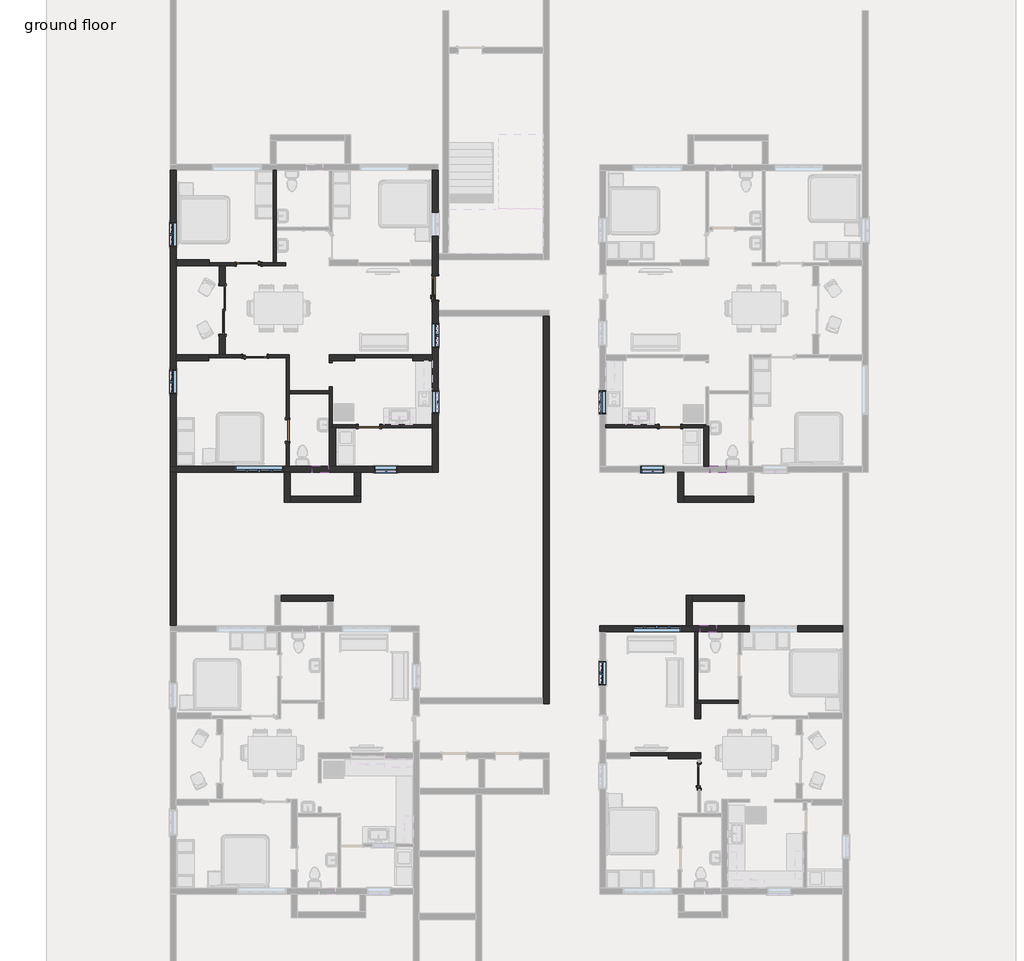
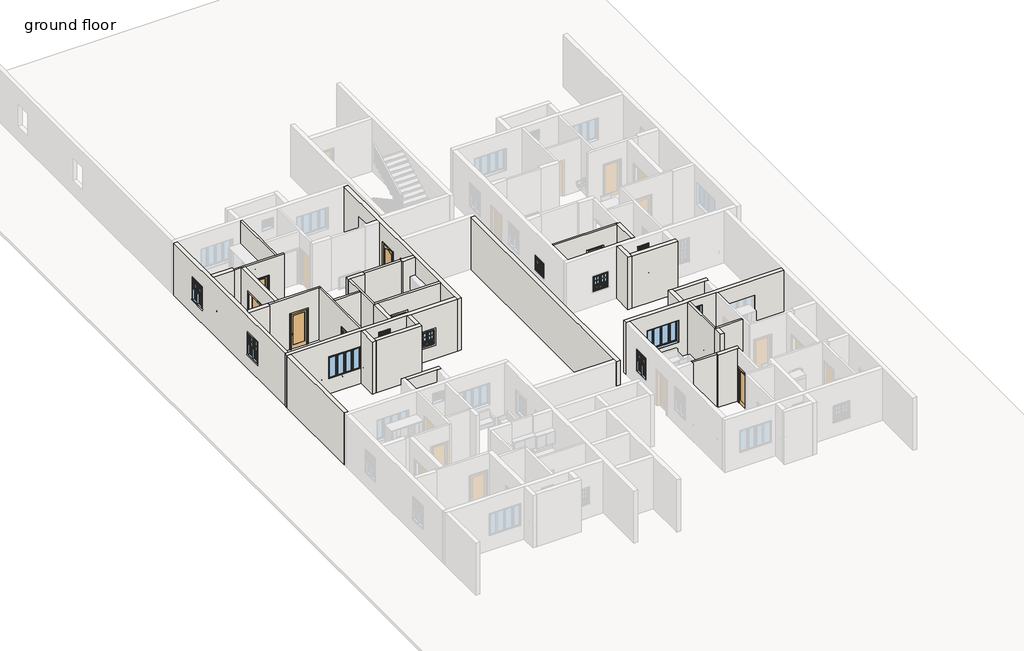
# One storey, part 6 of 16: 36 walls, 13 windows, 8 doors.
# Revit data of these elements (continued)
# Type "Window-Single-Hung-Double : 36\" x 52\"" (continued)
#   Exterior Trim Visibility [instance default] = yes
#   Define Thermal Properties by = 1
#   Bottom Muntin Visibility = yes
#   Muntin Pattern = Muntin Pattern_2x2 : Muntin Pattern_2x2
#   Interior Trim = Trim-Window-Interior-Flat : Picture Frame
#   Interior Trim Material = Wood - Stained
#   Exterior Trim Material = Clad - White
#   Exterior Trim = Trim-Window-Exterior-Flat : with Sill
#   Glass Panel Material = Glass
#   Exterior Frame Material = Clad - White
#   Interior Frame Material = Wood - Stained
#   Wall Closure = (empty or 0)
# Element 1 (IfcDoor, "36\" x 84\"")
#   Threshold Offset = 0' - 0 1/2"
#   Swing Angle = 90.00°
#   Door Offset = 0' - 0"
#   Threshold = yes
#   Exterior Trim = yes
#   Phase Created = New Construction
#   Materials on its faces: "Cherry", "Aluminum", "Glass"
# Element 2 (IfcDoor, "Door-Double-Sliding : 72\" x 84\"")
#   Phase Created = New Construction
#   Materials on its faces: "Paint - Sienna", "Wood - Birch - Solid Stained Light Low Gloss", "Glass"
# Elements 3, 4, 5 (IfcDoor, "Door-Interior-Single-1_Panel-Wood : 36\" x 84\"")
#   Swing Angle = 90.00°
#   Phase Created = New Construction
#   Materials on its faces: "Cherry", "Aluminum"
# Elements 6, 7, 8 (IfcDoor, "Single-Flush : 32\" x 84\"")
#   Phase Created = New Construction
#   Materials on its faces: "Door - Frame", "Door - Panel"
# Elements 9, 10, 11, 12, 13, 14, 15, 16, 17, 18, 19, 20, 21 (IfcWall, "Generic - 4.5\"")
#   Top Offset = 0' - 0"
#   Base Offset = 0' - 0"
#   wall height = 10' - 6"
#   Phase Created = New Construction
#   Base Constraint = ground floor
#   Top Constraint = 1st floor
#   Materials on its faces: "Default Wall"
# Element 22 (IfcWall, "Generic - 8\"")
#   Top Offset = 0' - 0"
#   Base Offset = 0' - 0"
#   wall height = 10' - 6"
#   Phase Created = New Construction
#   Base Constraint = ground floor
#   Top Constraint = 1st floor
#   Materials on its faces: "Default Wall"
# Elements 23, 24, 25, 26, 27, 28, 29, 30, 31, 32, 33, 34, 35, 36, 37, 38, 39, 40, 41, 42, 43, 44 (IfcWall, "Generic - 9\"")
#   Top Offset = 0' - 0"
#   Base Offset = 0' - 0"
#   wall height = 10' - 6"
#   Phase Created = New Construction
#   Base Constraint = ground floor
#   Top Constraint = 1st floor
#   Materials on its faces: "Default Wall"
# Element 45 (IfcWindow, "Window-Casement-Double-Awning : 34\" x 36\"")
#   Mark = "72"
#   Window Inset = 0' - 0"
#   Interior Wall Closure = 0' - 2 1/4"
#   Frame Extension = 0' - 0 1/4"
#   Exterior Wall Closure = 0' - 1 1/4"
#   Interior Trim Visibility = yes
#   Exterior Trim Visibility = yes
#   Phase Created = New Construction
#   Materials on its faces: "Wood - Stained", "Glass", "Clad - White"
# Element 46 (IfcWindow, "Window-Casement-Double-Awning : 34\" x 36\"")
#   Mark = "73"
#   Window Inset = 0' - 0"
#   Interior Wall Closure = 0' - 2 1/4"
#   Frame Extension = 0' - 0 1/4"
#   Exterior Wall Closure = 0' - 1 1/4"
#   Interior Trim Visibility = yes
#   Exterior Trim Visibility = yes
#   Phase Created = New Construction
#   Materials on its faces: "Wood - Stained", "Glass", "Clad - White"
# Element 47 (IfcWindow, "Window-Casement-Double-Awning : 34\" x 36\"")
#   Mark = "89"
#   Window Inset = 0' - 0"
#   Interior Wall Closure = 0' - 2 1/4"
#   Frame Extension = 0' - 0 1/4"
#   Exterior Wall Closure = 0' - 1 1/4"
#   Interior Trim Visibility = yes
#   Exterior Trim Visibility = yes
#   Phase Created = New Construction
#   Materials on its faces: "Wood - Stained", "Glass", "Clad - White"
# Element 48 (IfcWindow, "Window-Casement-Double-Awning : 34\" x 36\"")
#   Mark = "90"
#   Window Inset = 0' - 0"
#   Interior Wall Closure = 0' - 2 1/4"
#   Frame Extension = 0' - 0 1/4"
#   Exterior Wall Closure = 0' - 1 1/4"
#   Interior Trim Visibility = yes
#   Exterior Trim Visibility = yes
#   Phase Created = New Construction
#   Materials on its faces: "Wood - Stained", "Glass", "Clad - White"
# Element 49 (IfcWindow, "Window-Casement-Multi-Sash-Horizontal : 72\" x 53\"")
#   Mark = "24"
#   Window Inset = 0' - 0 5/8"
#   Frame Gap 3 = 0' - 1 83/128"
#   Frame Gap 2 = 0' - 0 5/8"
#   Phase Created = New Construction
#   Materials on its faces: "Metal - Aluminum", "Glass"
# Element 50 (IfcWindow, "Window-Casement-Multi-Sash-Horizontal : 72\" x 53\"")
#   Mark = "40"
#   Window Inset = 0' - 0 5/8"
#   Frame Gap 3 = 0' - 1 83/128"
#   Frame Gap 2 = 0' - 0 5/8"
#   Phase Created = New Construction
#   Materials on its faces: "Metal - Aluminum", "Glass"
# Element 51 (IfcWindow, "Window-Louvers : 24\" x 24\"")
#   Mark = "95"
#   Blade Width = 1' - 10 1/2"
#   Phase Created = New Construction
#   Materials on its faces: "Birch"
# Element 52 (IfcWindow, "Window-Louvers : 24\" x 24\"")
#   Mark = "96"
#   Blade Width = 1' - 10 1/2"
#   Phase Created = New Construction
#   Materials on its faces: "Birch"
# Element 53 (IfcWindow, "Window-Louvers : 24\" x 24\"")
#   Mark = "110"
#   Blade Width = 1' - 10 1/2"
#   Phase Created = New Construction
#   Materials on its faces: "Birch"
# Element 54 (IfcWindow, "Window-Single-Hung-Double : 36\" x 52\"")
#   Mark = "48"
#   Window Inset = 0' - 0"
#   Interior Wall Closure = 0' - 1 1/2"
#   Frame Extension = 0' - 1 1/4"
#   Exterior Wall Closure = 0' - 0 1/2"
#   Interior Trim Visibility = yes
#   Indicator Visibility = yes
#   Exterior Trim Visibility = yes
#   Phase Created = New Construction
#   Materials on its faces: "Wood - Stained", "Glass", "Clad - White"
# Element 55 (IfcWindow, "Window-Single-Hung-Double : 36\" x 52\"")
#   Mark = "64"
#   Window Inset = 0' - 0"
#   Interior Wall Closure = 0' - 1 1/2"
#   Frame Extension = 0' - 1 1/4"
#   Exterior Wall Closure = 0' - 0 1/2"
#   Interior Trim Visibility = yes
#   Indicator Visibility = yes
#   Exterior Trim Visibility = yes
#   Phase Created = New Construction
#   Materials on its faces: "Wood - Stained", "Glass", "Clad - White"
# Element 56 (IfcWindow, "Window-Single-Hung-Double : 36\" x 52\"")
#   Mark = "65"
#   Window Inset = 0' - 0"
#   Interior Wall Closure = 0' - 1 1/2"
#   Frame Extension = 0' - 1 1/4"
#   Exterior Wall Closure = 0' - 0 1/2"
#   Interior Trim Visibility = yes
#   Indicator Visibility = yes
#   Exterior Trim Visibility = yes
#   Phase Created = New Construction
#   Materials on its faces: "Wood - Stained", "Glass", "Clad - White"
# Element 57 (IfcWindow, "Window-Single-Hung-Double : 36\" x 52\"")
#   Mark = "66"
#   Window Inset = 0' - 0"
#   Interior Wall Closure = 0' - 1 1/2"
#   Frame Extension = 0' - 1 1/4"
#   Exterior Wall Closure = 0' - 0 1/2"
#   Interior Trim Visibility = yes
#   Indicator Visibility = yes
#   Exterior Trim Visibility = yes
#   Phase Created = New Construction
#   Materials on its faces: "Wood - Stained", "Glass", "Clad - White"
# Materials
#   "Cherry": class "Wood", colour RGB 226 177 128, transparency 0, Description = "Prunus Serotina", Cost = 0
#   "Glass": class "Glass", colour RGB 0 128 192, transparency 0.75, Description = "Soda Lime Glass", Cost = 0
#   "Aluminum": class "Metal", colour RGB 247 247 247, transparency 0, Description = "Aluminum 6061", Cost = 0
#   "Wood - Birch - Solid Stained Light Low Gloss": class "Wood", colour RGB 210 159 95, transparency 0, Cost = 0
#   "Paint - Sienna": colour RGB 118 70 51, transparency 0, Cost = 0
#   "Door - Panel": class "Wood", colour RGB 210 159 95, transparency 0, Cost = 0
#   "Door - Frame": colour RGB 118 70 51, transparency 0, Cost = 0
#   "Wood - Stained": class "Wood", colour RGB 224 178 126, transparency 0, Cost = 0
#   "Clad - White": class "Wood", colour RGB 242 242 238, transparency 0, Cost = 0
#   "Metal - Aluminum": class "Metal", colour RGB 247 247 247, transparency 0
#   "Birch": class "Wood", colour RGB 224 178 126, transparency 0, Description = "Betula Alleghaniensis", Cost = 0
#   "Default Wall": colour RGB 128 128 128, transparency 0, Cost = 0
